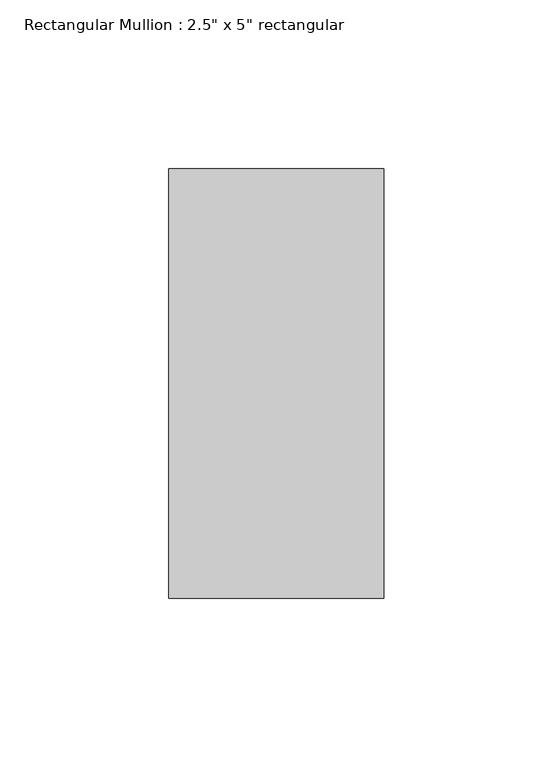
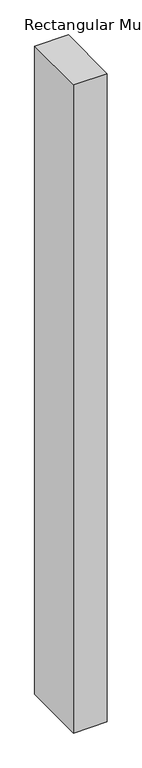
"""IFC4 building model written with IfcOpenShell, lengths in millimetres: member geometry."""

from ifc_helpers import new_model, si_unit, frame, origin, place, context, project, spatial, polyline, outline, extrude, source, transform, mapped, element, save


def member_2a4e9e33(model_context):
    return source(origin(), model_context, "Body", "SweptSolid", [
        extrude(outline(polyline([(0.0, 63.5), (0.0, -63.5), (-63.5, -63.5), (-63.5, 63.5), (0.0, 63.5)])), frame((0.0, 0.0, -1293.8688597), z_axis=(0.0, 0.0, 1.0), x_axis=(1.0, 0.0, 0.0)), (0.0, 0.0, 1.0), 1293.8688597),
    ])


if __name__ == "__main__":
    model = new_model("IFC4")
    model_context = context("Model", 3, world=origin())
    ifc_project = project(units=[si_unit("LENGTHUNIT", "METRE", prefix="MILLI")], contexts=[model_context])
    site = spatial("IfcSite", under=ifc_project)
    building = spatial("IfcBuilding", under=site)
    placement = place(None, origin())
    member_shape = member_2a4e9e33(model_context)
    element("IfcMember", 1, ObjectType="Rectangular Mullion : 2.5\" x 5\" rectangular", at=placement, inside=building, context=model_context, shape_type="MappedRepresentation", body=[
        mapped(member_shape, transform((0.0, 0.0, 0.0), x_axis=(1.0, 0.0, 0.0), y_axis=(0.0, 1.0, 0.0), z_axis=(0.0, 0.0, 1.0))),
    ])
    save(model, "model.ifc")

# Revit data of these elements
# Type "Rectangular Mullion : 2.5\" x 5\" rectangular"
#   built-in parameter 1007304 = 0.416667 (stored number, unit not read)
#   built-in parameter 1007301 = 0.104167 (stored number, unit not read)
#   built-in parameter 1007300 = 0.104167 (stored number, unit not read)
# Element 1 (IfcMember, "Rectangular Mullion : 2.5\" x 5\" rectangular")
#   Materials on its faces: "metal black"
# Materials
#   "metal black": class "Generic", colour RGB 120 120 120, transparency 0, Cost = 0
